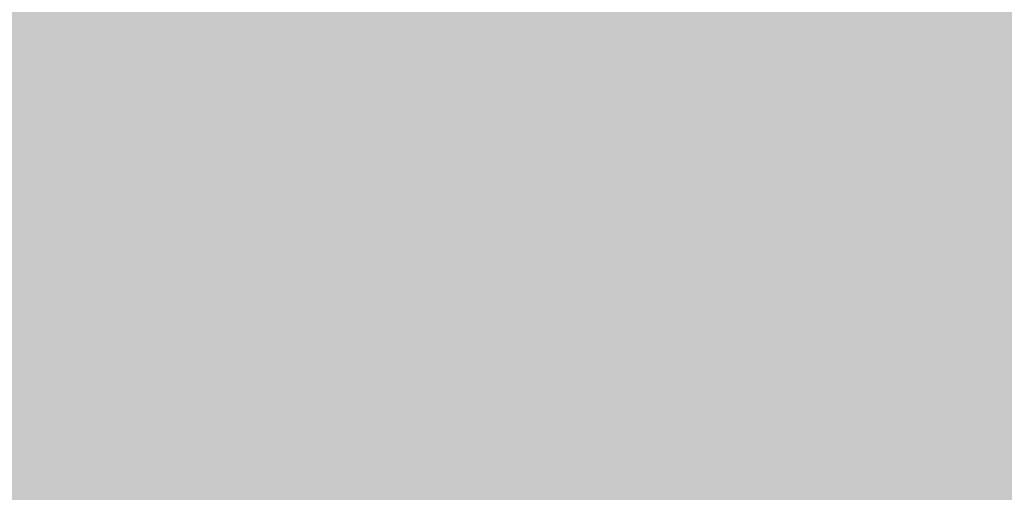
# Model space of a CAD drawing. Units: inches. Extents: x 2083 to 3317, y 1141 to 2115.
# Tile 131 of 256: x 3119.674 to 3123.979, y 1265.165 to 1267.234. Entities that reach past the tile are written whole.
import ezdxf

# ---------------------------------------------------------------- set-up
doc = ezdxf.new("R2010")
doc.units = ezdxf.units.IN
doc.layers.add('A-ANNO-DIMS', color=2, linetype='Continuous', lineweight=18)
doc.layers.add('A-WALL-PATT', color=251, linetype='Continuous', lineweight=13, true_color=0x636466)
doc.styles.get("Standard").update_dxf_attribs({"font": 'arial.ttf'})
doc.dimstyles.new('ISO-25', dxfattribs={"dimtxt": 12, "dimasz": 12, "dimexe": 1.25, "dimexo": 0.625, "dimtad": 1, "dimlunit": 3, "dimtxsty": 'Standard', "dimcen": 2.5, "dimadec": 0, "dimazin": 0, "dimtfac": 1, "dimtmove": 0, "dimatfit": 3, "dimfxl": 1, "dimarcsym": 0})

# ---------------------------------------------------------------- blocks, each defined once
blk = doc.blocks.new('*D26')
at = {"layer": 'A-ANNO-DIMS', "color": 0, "lineweight": -2, "transparency": 16777216}
for p, q in [((3088.9858, 1274.9151), (3088.9858, 1270.952)), ((3111.24, 1274.9151), (3111.24, 1270.952)), ((3076.9858, 1272.202), (2840.2624, 1272.202)), ((3111.24, 1272.202), (3088.9858, 1272.202)), ((3123.24, 1272.202), (3135.24, 1272.202))]:
    blk.add_line(p, q, dxfattribs=at)
at = {"layer": 'A-ANNO-DIMS', "color": 0, "transparency": 16777216}
for points in [[(3076.9858, 1274.202), (3076.9858, 1270.202), (3088.9858, 1272.202)], [(3123.24, 1274.202), (3123.24, 1270.202), (3111.24, 1272.202)]]:
    blk.add_solid(points, dxfattribs=at)
at = {"layer": 'Defpoints', "color": 0, "transparency": 16777216}
for p in [(3088.9858, 1275.5401), (3111.24, 1275.5401), (3088.9858, 1272.202)]:
    blk.add_point(p, dxfattribs=at)
at = {"layer": 'A-ANNO-DIMS', "color": 0, "transparency": 16777216, "insert": (2952.6241, 1279.0316), "char_height": 12, "attachment_point": 5}
blk.add_mtext('NIGHTSTAND 1\'-10 1/2" TYP.', dxfattribs=at)
blk = doc.blocks.new('*D27')
at = {"layer": 'A-ANNO-DIMS', "color": 0, "lineweight": -2, "transparency": 16777216}
for p, q in [((3114.5782, 1309.7943), (3114.5782, 1321.7943)), ((3111.865, 1297.7943), (3115.8282, 1297.7943)), ((3114.5782, 1297.7943), (3114.5782, 1275.5401)), ((3111.865, 1275.5401), (3115.8282, 1275.5401)), ((3114.5782, 1263.5401), (3114.5782, 1140.9886))]:
    blk.add_line(p, q, dxfattribs=at)
at = {"layer": 'A-ANNO-DIMS', "color": 0, "transparency": 16777216}
for points in [[(3112.5782, 1309.7943), (3116.5782, 1309.7943), (3114.5782, 1297.7943)], [(3112.5782, 1263.5401), (3116.5782, 1263.5401), (3114.5782, 1275.5401)]]:
    blk.add_solid(points, dxfattribs=at)
at = {"layer": 'Defpoints', "color": 0, "transparency": 16777216}
for p in [(3111.24, 1297.7943), (3111.24, 1275.5401), (3114.5782, 1275.5401)]:
    blk.add_point(p, dxfattribs=at)
at = {"layer": 'A-ANNO-DIMS', "color": 0, "transparency": 16777216, "insert": (3107.7485, 1196.2643), "char_height": 12, "attachment_point": 5, "rotation": 90}
blk.add_mtext('1\'-10 1/2" TYP.', dxfattribs=at)

msp = doc.modelspace()

# ---------------------------------------------------------------- hatches: boundary and pattern name
at = {"layer": 'A-WALL-PATT'}
h = msp.add_hatch(color=256, dxfattribs=at)
h.dxf.hatch_style = 1
h.paths.add_polyline_path([(3126.9598, 2020.7614), (2748.9598, 2020.7614), (2604.9598, 2020.7614), (2226.9598, 2020.7614), (2226.9598, 1702.7614), (2466.9598, 1702.7614), (2466.9598, 1582.7614), (2418.9598, 1582.7614), (2418.9598, 1477.7614), (2226.9598, 1477.7614), (2226.9598, 1263.2614), (2544.9598, 1263.2614), (2544.9598, 1411.7614), (2604.9598, 1411.7614), (2685.9598, 1411.7614), (2685.9598, 1420.7614), (2604.9598, 1420.7614), (2604.9598, 1573.7614), (2604.9598, 1702.7614), (2604.9598, 2011.7614), (2748.9598, 2011.7614), (2748.9598, 1702.7614), (2862.9598, 1702.7614), (2862.9598, 1621.7614), (2871.9598, 1621.7614), (2871.9598, 1702.7614), (2883.9598, 1702.7614), (2883.9598, 1706.9395, -0.026459), (2883.9598, 1711.7614), (2757.9598, 1711.7614), (2757.9598, 1807.7614), (2787.9598, 1807.7614), (2787.9598, 1812.2614), (2757.9598, 1812.2614), (2757.9598, 2011.7614), (2877.9598, 2011.7614), (2877.9598, 1812.2614), (2847.9598, 1812.2614), (2847.9598, 1807.7614), (2889.8357, 1807.7614), (2889.8357, 1812.2614), (2882.4598, 1812.2614), (2882.4598, 2011.7614), (3117.9598, 2011.7614), (3117.9598, 1812.2614), (2937.8357, 1812.2614), (2937.8357, 1807.7614), (2995.7098, 1807.7614), (2995.7098, 1796.1177), (3000.2098, 1796.1177), (3000.2098, 1807.7614), (3117.9598, 1807.7614), (3117.9598, 1711.7614), (3000.2098, 1711.7614), (3000.2098, 1760.1177), (2998.5727, 1760.1177, -0.020711), (2995.7098, 1760.1177), (2995.7098, 1711.7614), (2931.9598, 1711.7614), (2931.9598, 1702.7614), (3126.9598, 1702.7614)])
h.paths.add_polyline_path([(2471.4598, 2011.7614), (2471.4598, 1810.0114), (2462.7169, 1810.0114), (2462.7169, 1805.5114), (2505.9598, 1805.5114), (2505.9598, 1810.0114), (2475.9598, 1810.0114), (2475.9598, 2011.7614), (2595.9598, 2011.7614), (2595.9598, 1810.0114), (2565.9598, 1810.0114), (2565.9598, 1805.5114), (2595.9598, 1805.5114), (2595.9598, 1711.7614), (2235.9598, 1711.7614), (2235.9598, 1805.5114), (2353.7098, 1805.5114), (2353.7098, 1796.0542), (2358.2098, 1796.0542), (2358.2098, 1805.5114), (2414.7169, 1805.5114), (2414.7169, 1810.0114), (2235.9598, 1810.0114), (2235.9598, 2011.7614)], flags=16)
h.paths.add_polyline_path([(2270.2047, 1994.61), (2270.2047, 1970.61), (2246.2047, 1970.61), (2246.2047, 1994.61)], flags=0)
edge = h.paths.add_edge_path(flags=0)
edge.add_ellipse((2332.0274, 1899.7982), major_axis=(-3.043, 3.043), ratio=0.168252, start_angle=-161.3322, end_angle=-156.3071, ccw=False)
edge.add_ellipse((2333.082, 1898.7435), major_axis=(-1.0546, 1.0546), ratio=0.453532, start_angle=-123.371, end_angle=-94.1591)
edge = h.paths.add_edge_path(flags=0)
edge.add_ellipse((2332.0274, 1968.8763), major_axis=(3.043, 3.043), ratio=0.168252, start_angle=18.6678, end_angle=23.6929)
edge.add_spline(control_points=[(2332.9256, 1970.6911), (2332.2268, 1970.3361), (2330.8937, 1969.6589), (2328.4131, 1970.9321), (2327.2039, 1967.7487), (2324.7096, 1969.9556), (2322.5328, 1967.0124), (2320.0128, 1971.2958), (2317.6803, 1968.1578), (2316.0405, 1967.102), (2315.4269, 1966.8096)], knot_values=[0, 0, 0, 0, 2.267059, 4.324559, 6.685584, 8.878641, 11.121502, 14.300359, 17.755284, 19.732645, 19.732645, 19.732645, 19.732645], degree=3, periodic=0)
edge.add_ellipse((2332.0274, 1968.8763), major_axis=(3.043, 3.043), ratio=0.168252, start_angle=18.6678, end_angle=23.6929, ccw=False)
edge.add_ellipse((2333.082, 1969.9309), major_axis=(1.0546, 1.0546), ratio=0.453532, start_angle=56.629, end_angle=85.8409, ccw=False)
edge = h.paths.add_edge_path(flags=0)
edge.add_spline(control_points=[(2296.4283, 1967.9879), (2293.6278, 1965.3363), (2287.7036, 1959.7271), (2299.7439, 1949.9957), (2294.5326, 1935.6685), (2290.5732, 1920.6035), (2293.3941, 1909.9737), (2296.1854, 1904.9665)], knot_values=[0.099185, 0.099185, 0.099185, 0.099185, 0.345301, 0.619822, 0.982653, 1.386093, 1.810555, 1.810555, 1.810555, 1.810555], degree=3, periodic=0)
edge.add_spline(control_points=[(2296.1854, 1904.9665), (2297.3836, 1902.6193), (2298.001, 1901.9493), (2298.553, 1901.4682)], knot_values=[0.006246, 0.006246, 0.006246, 0.006246, 0.055476, 0.055476, 0.055476, 0.055476], degree=3, periodic=0)
edge.add_spline(control_points=[(2298.553, 1901.4682), (2297.2586, 1900.9232), (2295.2253, 1900.2321), (2293.0602, 1900.6142), (2292.1014, 1900.7884), (2292.0896, 1900.7906)], knot_values=[0.312835, 0.312835, 0.312835, 0.312835, 0.40178, 0.474987, 0.475903, 0.475903, 0.475903, 0.475903], degree=3, periodic=0)
edge.add_arc((2292.7936, 1904.6641), 3.937, 215.4209, 259.6982, ccw=False)
edge.add_spline(control_points=[(2289.5853, 1902.3823), (2289.4767, 1902.5351), (2289.3685, 1902.688), (2289.2609, 1902.8412)], knot_values=[0.102872, 0.102872, 0.102872, 0.102872, 0.116896, 0.116896, 0.116896, 0.116896], degree=3, periodic=0)
edge.add_spline(control_points=[(2289.2609, 1902.8412), (2288.6866, 1902.5502), (2287.64, 1902.0199), (2285.8813, 1901.874), (2283.853, 1901.5044), (2281.72, 1899.7105), (2278.467, 1899.4929), (2276.1571, 1901.8832), (2272.259, 1899.8041), (2267.7776, 1901.8432), (2262.2439, 1900.184), (2257.4149, 1901.7821), (2254.3184, 1900.7261), (2253.1783, 1900.3373)], knot_values=[0, 0, 0, 0, 1.907977, 3.477176, 5.261074, 7.972851, 11.680248, 13.717921, 16.939592, 22.789562, 27.502503, 33.595215, 37.145618, 37.145618, 37.145618, 37.145618], degree=3, periodic=0)
edge.add_line((2253.1783, 1900.3373), (2250.2442, 1902.8412))
edge.add_line((2250.2442, 1902.8412), (2250.2442, 1965.8333))
edge.add_line((2250.2442, 1965.8333), (2253.1783, 1968.3371))
edge.add_spline(control_points=[(2253.1783, 1968.3371), (2254.3184, 1967.9483), (2257.4149, 1966.8924), (2262.2439, 1968.4904), (2267.7776, 1966.8313), (2271.5267, 1968.5372), (2273.8759, 1967.8283), (2274.2067, 1967.7276)], knot_values=[0, 0, 0, 0, 0.09018, 0.244935, 0.364644, 0.513233, 0.537855, 0.537855, 0.537855, 0.537855], degree=3, periodic=0)
edge.add_arc((2274.3529, 1963.7933), 3.937, 72.0511, 92.1279, ccw=False)
edge.add_arc((2281.2969, 1985.23), 18.5963, 252.05113, 288.56572)
edge.add_arc((2292.3167, 1956.0289), 12.6461, 71.02679, 113.77822, ccw=False)
edge = h.paths.add_edge_path(flags=0)
edge.add_spline(control_points=[(2274.8994, 1951.8562), (2275.0662, 1951.6166), (2275.2327, 1951.3766), (2275.398, 1951.1359)], knot_values=[1.409916, 1.409916, 1.409916, 1.409916, 1.43159, 1.43159, 1.43159, 1.43159], degree=3, periodic=0)
edge.add_spline(control_points=[(2275.398, 1951.1359), (2275.7921, 1950.5619), (2276.1792, 1949.9838), (2276.5455, 1949.3971)], knot_values=[1.358238, 1.358238, 1.358238, 1.358238, 1.409916, 1.409916, 1.409916, 1.409916], degree=3, periodic=0)
edge.add_line((2276.5455, 1949.3971), (2277.4373, 1947.8622))
edge.add_spline(control_points=[(2277.4373, 1947.8622), (2276.3038, 1945.6731), (2274.6397, 1942.4269), (2274.6316, 1938.0939), (2272.7991, 1930.8515), (2274.3564, 1943.897), (2275.9477, 1947.9234), (2276.5455, 1949.3971)], knot_values=[0.005632, 0.005632, 0.005632, 0.005632, 0.186014, 0.266002, 0.357087, 0.59639, 0.739732, 0.739732, 0.739732, 0.739732], degree=3, periodic=0)
edge.add_spline(control_points=[(2276.5455, 1949.3971), (2276.1792, 1949.9838), (2275.7921, 1950.5619), (2275.398, 1951.1359)], knot_values=[1.358238, 1.358238, 1.358238, 1.358238, 1.409916, 1.409916, 1.409916, 1.409916], degree=3, periodic=0)
edge.add_spline(control_points=[(2275.398, 1951.1359), (2274.9425, 1950.0805), (2274.2078, 1948.0253), (2273.9346, 1944.8515), (2272.4685, 1937.6275), (2273.4662, 1945.6965), (2274.7006, 1951.0595), (2274.8994, 1951.8562)], knot_values=[0.104364, 0.104364, 0.104364, 0.104364, 0.189636, 0.269624, 0.36071, 0.600013, 0.644622, 0.644622, 0.644622, 0.644622], degree=3, periodic=0)
h.paths.add_polyline_path([(2269.1675, 1963.1276, -0.357527), (2268.1706, 1960.9764, -0.092561), (2268.1706, 1939.4363, -0.357527), (2269.1675, 1937.2851, -0.357527), (2267.0163, 1938.282, -0.164785), (2254.6856, 1938.282, -0.357527), (2252.5344, 1937.2851, -0.357527), (2253.5313, 1939.4363, -0.092561), (2253.5313, 1960.9764, -0.357527), (2252.5344, 1963.1276, -0.357527), (2254.6856, 1962.1307, -0.164785), (2267.0163, 1962.1307, -0.357527)], flags=0)
h.paths.add_polyline_path([(2248.8741, 1967.8018), (2248.8741, 1957.0277), (2249.4578, 1957.0277), (2249.4578, 1911.6468), (2248.8741, 1911.6468), (2248.8741, 1900.8727), (2246.5119, 1900.8727, 0.197327), (2244.1497, 1902.4569), (2244.1497, 1966.2176, 0.197327), (2246.5119, 1967.8018)], flags=0)
h.paths.add_polyline_path([(2269.1675, 1931.3893, -0.357527), (2268.1706, 1929.2381, -0.092561), (2268.1706, 1907.6981, -0.357527), (2269.1675, 1905.5469, -0.357527), (2267.0163, 1906.5438, -0.164785), (2254.6856, 1906.5438, -0.357527), (2252.5344, 1905.5469, -0.357527), (2253.5313, 1907.6981, -0.092561), (2253.5313, 1929.2381, -0.357527), (2252.5344, 1931.3893, -0.357527), (2254.6856, 1930.3925, -0.164785), (2267.0163, 1930.3925, -0.357527)], flags=0)
edge = h.paths.add_edge_path(flags=0)
edge.add_spline(control_points=[(2276.1969, 1906.7237), (2276.1681, 1909.0289), (2276.114, 1913.3719), (2270.5984, 1924.925), (2273.9052, 1919.0128), (2275.9217, 1916.2621), (2275.4746, 1912.4021), (2277.2579, 1910.3806), (2276.696, 1908.225), (2276.6462, 1906.813), (2276.6178, 1906.0084)], knot_values=[0, 0, 0, 0, 8.61026, 16.221274, 18.843057, 23.804898, 27.440828, 29.356102, 31.203478, 33.650687, 33.650687, 33.650687, 33.650687], degree=3, periodic=0)
edge.add_spline(control_points=[(2276.6178, 1906.0084), (2276.6233, 1905.6241), (2276.4977, 1904.6287), (2275.4418, 1903.8547), (2274.9373, 1903.0804), (2274.8591, 1902.8412)], knot_values=[0.156488, 0.156488, 0.156488, 0.156488, 0.184398, 0.231376, 0.250598, 0.250598, 0.250598, 0.250598], degree=3, periodic=0)
edge.add_line((2274.8591, 1902.8412), (2276.506, 1902.8412))
edge.add_spline(control_points=[(2276.506, 1902.8412), (2276.7883, 1903.0849), (2277.6651, 1904.1252), (2278.2495, 1904.3407), (2277.6539, 1908.5274), (2278.1557, 1906.2278), (2278.1005, 1905.2859), (2278.8467, 1904.069), (2277.8568, 1903.4149), (2277.8742, 1902.991), (2277.9036, 1902.8412)], knot_values=[0.059574, 0.059574, 0.059574, 0.059574, 0.080753, 0.103741, 0.16972, 0.176036, 0.207137, 0.240474, 0.262341, 0.27366, 0.27366, 0.27366, 0.27366], degree=3, periodic=0)
edge.add_line((2277.9036, 1902.8412), (2280.0298, 1902.8412))
edge.add_spline(control_points=[(2280.0298, 1902.8412), (2279.8882, 1903.0884), (2279.4993, 1903.9816), (2280.1523, 1905.9393), (2278.1036, 1909.6578), (2279.7624, 1907.1853), (2280.3279, 1904.8749), (2280.4851, 1903.4896), (2281.4633, 1903.2494), (2281.7583, 1902.9365), (2281.834, 1902.8412)], knot_values=[0.013856, 0.013856, 0.013856, 0.013856, 0.034874, 0.088867, 0.107879, 0.126738, 0.158714, 0.193757, 0.217487, 0.226722, 0.226722, 0.226722, 0.226722], degree=3, periodic=0)
edge.add_spline(control_points=[(2281.834, 1902.8412), (2281.7875, 1902.8267), (2281.647, 1902.783), (2281.3955, 1902.8595), (2281.0881, 1902.9852), (2280.7207, 1903.0609), (2280.3335, 1903.0257), (2280.1248, 1902.8989), (2280.0298, 1902.8412)], knot_values=[0, 0, 0, 0, 0.14413, 0.435517, 0.749276, 1.153046, 1.548371, 1.878348, 1.878348, 1.878348, 1.878348], degree=3, periodic=0)
edge.add_line((2280.0298, 1902.8412), (2277.9036, 1902.8412))
edge.add_spline(control_points=[(2277.9036, 1902.8412), (2277.8929, 1902.7959), (2277.8654, 1902.6796), (2277.6075, 1902.6875), (2277.2741, 1902.8007), (2276.8379, 1902.6198), (2276.5838, 1902.7893), (2276.506, 1902.8412)], knot_values=[0, 0, 0, 0, 0.127189, 0.326199, 0.628009, 1.24357, 1.515331, 1.515331, 1.515331, 1.515331], degree=3, periodic=0)
edge.add_line((2276.506, 1902.8412), (2274.8591, 1902.8412))
edge.add_spline(control_points=[(2274.8591, 1902.8412), (2274.8144, 1902.8986), (2274.7251, 1903.0134), (2274.4935, 1903.119), (2274.2443, 1902.9605), (2273.9371, 1903.1849), (2273.614, 1902.9831), (2273.4083, 1902.883), (2273.3223, 1902.8412)], knot_values=[0, 0, 0, 0, 0.21843, 0.436957, 0.687977, 0.990379, 1.398396, 1.69185, 1.69185, 1.69185, 1.69185], degree=3, periodic=0)
edge.add_spline(control_points=[(2273.3223, 1902.8412), (2273.6167, 1903.4457), (2274.274, 1904.5383), (2276.0272, 1904.5737), (2276.207, 1906.5836), (2276.1969, 1906.7237)], knot_values=[0.012227, 0.012227, 0.012227, 0.012227, 0.059472, 0.106218, 0.134458, 0.134458, 0.134458, 0.134458], degree=3, periodic=0)
h.paths.add_polyline_path([(2270.7761, 1897.7898), (2270.7761, 1873.7898), (2246.7761, 1873.7898), (2246.7761, 1897.7898)], flags=0)
h.paths.add_polyline_path([(2353.7098, 1760.0051), (2353.7098, 1760.0542), (2358.2098, 1760.0542, -0.033729)], flags=0)
h.paths.add_polyline_path([(2321.8191, 1737.5292), (2341.9953, 1737.5292, -0.414214), (2343.2033, 1736.3212), (2343.2033, 1721.0206, -0.414214), (2341.9953, 1719.8127), (2321.8191, 1719.8127, -0.414214), (2320.6112, 1721.0206), (2320.6112, 1736.3212, -0.414214)], flags=0)
h.paths.add_polyline_path([(2324.235, 1736.3212), (2339.5794, 1736.3212, -0.414214), (2341.9953, 1733.9053), (2341.9953, 1725.4497, -0.414214), (2339.5794, 1723.0338), (2333.6806, 1723.0338), (2333.8453, 1722.0455, -0.870646), (2335.4254, 1721.8259, -0.767327), (2333.9227, 1721.4232), (2331.291, 1721.4232, -0.767327), (2329.7883, 1721.8259, -0.870646), (2331.3684, 1722.0455), (2331.5331, 1723.0338), (2324.235, 1723.0338, -0.414214), (2321.8191, 1725.4497), (2321.8191, 1733.9053, -0.414214)], flags=0)
h.paths.add_polyline_path([(2570.4838, 1928.6154), (2589.6838, 1928.6154), (2590.1688, 1928.6154), (2590.1688, 1904.9934), (2570.4838, 1904.9934)], flags=0)
h.paths.add_polyline_path([(2574.4473, 1927.2638, -1), (2572.8288, 1927.2638, -1)], flags=0)
h.paths.add_polyline_path([(2573.0899, 1926.9409), (2573.925, 1927.776), (2574.1477, 1927.5533), (2573.3126, 1926.7182)], flags=0)
h.paths.add_polyline_path([(2578.7791, 1919.7296, -1), (2571.5917, 1919.7296, -1)], flags=0)
h.paths.add_polyline_path([(2578.3854, 1919.7296, -1), (2571.9854, 1919.7296, -1)], flags=0)
h.paths.add_polyline_path([(2331.5958, 1729.4762, -1), (2333.618, 1729.4762, -1)], flags=0)
h.paths.add_polyline_path([(2578.0342, 1927.2638, -1), (2576.4157, 1927.2638, -1)], flags=0)
h.paths.add_polyline_path([(2576.6889, 1927.5311), (2576.9116, 1927.7538), (2577.7467, 1926.9186), (2577.524, 1926.6959)], flags=0)
h.paths.add_polyline_path([(2578.1391, 1909.8595, -1), (2572.2317, 1909.8595, -1)], flags=0)
h.paths.add_polyline_path([(2577.7454, 1909.8595, -1), (2572.6254, 1909.8595, -1)], flags=0)
h.paths.add_polyline_path([(2583.7977, 1927.2638, -1), (2582.1792, 1927.2638, -1)], flags=0)
h.paths.add_polyline_path([(2582.7186, 1927.7538), (2583.5538, 1926.9186), (2583.3311, 1926.6959), (2582.4959, 1927.5311)], flags=0)
h.paths.add_polyline_path([(2582.4959, 1927.5311), (2582.7186, 1927.7538), (2583.5538, 1926.9186), (2583.3311, 1926.6959)], flags=0)
h.paths.add_polyline_path([(2587.7391, 1920.5296, -1), (2581.8317, 1920.5296, -1)], flags=0)
h.paths.add_polyline_path([(2587.3454, 1920.5296, -1), (2582.2254, 1920.5296, -1)], flags=0)
h.paths.add_polyline_path([(2587.3846, 1927.2638, -1), (2585.7661, 1927.2638, -1)], flags=0)
h.paths.add_polyline_path([(2586.082, 1926.9802), (2586.9172, 1927.8154), (2587.1399, 1927.5927), (2586.3047, 1926.7575)], flags=0)
h.paths.add_polyline_path([(2588.3791, 1910.6595, -1), (2581.1917, 1910.6595, -1)], flags=0)
h.paths.add_polyline_path([(2587.9854, 1910.6595, -1), (2581.5854, 1910.6595, -1)], flags=0)
h.paths.add_polyline_path([(2417.1677, 1729.4779), (2437.3439, 1729.4779, -0.414214), (2438.5519, 1728.2699), (2438.5519, 1712.9693, -0.414214), (2437.3439, 1711.7614), (2417.1677, 1711.7614, -0.414214), (2415.9598, 1712.9693), (2415.9598, 1728.2699, -0.414214)], flags=0)
h.paths.add_polyline_path([(2419.5836, 1728.2699), (2434.928, 1728.2699, -0.414214), (2437.3439, 1725.8541), (2437.3439, 1717.3984, -0.414214), (2434.928, 1714.9825), (2429.0292, 1714.9825), (2429.1939, 1713.9942, -0.870646), (2430.774, 1713.7746, -0.767327), (2429.2713, 1713.372), (2426.6396, 1713.372, -0.767327), (2425.1369, 1713.7746, -0.870646), (2426.717, 1713.9942), (2426.8817, 1714.9825), (2419.5836, 1714.9825, -0.414214), (2417.1677, 1717.3984), (2417.1677, 1725.8541, -0.414214)], flags=0)
h.paths.add_polyline_path([(2419.5836, 1728.2699), (2434.928, 1728.2699, -0.414214), (2437.3439, 1725.8541), (2437.3439, 1717.3984, -0.414214), (2434.928, 1714.9825), (2429.0292, 1714.9825), (2428.3581, 1719.009), (2427.5528, 1719.009), (2426.8817, 1714.9825), (2419.5836, 1714.9825, -0.414214), (2417.1677, 1717.3984), (2417.1677, 1725.8541, -0.414214)], flags=0)
h.paths.add_polyline_path([(2426.9444, 1721.4249, -1), (2428.9666, 1721.4249, -1)], flags=0)
h.paths.add_polyline_path([(2475.9598, 1702.7614), (2595.9598, 1702.7614), (2595.9598, 1582.7614), (2475.9598, 1582.7614)], flags=16)
h.paths.add_polyline_path([(2427.9598, 1573.7614), (2595.9598, 1573.7614), (2595.9598, 1468.7614), (2595.9598, 1420.7614), (2384.4598, 1420.7614), (2384.4598, 1468.7614), (2427.9598, 1468.7614)], flags=16)
h.paths.add_polyline_path([(2379.9598, 1468.7614), (2379.9598, 1420.7614), (2235.9598, 1420.7614), (2235.9598, 1468.7614)], flags=16)
h.paths.add_polyline_path([(2317.816, 1466.6958), (2337.9922, 1466.6958, -0.414214), (2339.2002, 1465.4878), (2339.2002, 1450.1872, -0.414214), (2337.9922, 1448.9792), (2317.816, 1448.9792, -0.414214), (2316.6081, 1450.1872), (2316.6081, 1465.4878, -0.414214)], flags=0)
h.paths.add_polyline_path([(2320.2319, 1465.4878), (2335.5763, 1465.4878, -0.414214), (2337.9922, 1463.0719), (2337.9922, 1454.6163, -0.414214), (2335.5763, 1452.2004), (2329.6775, 1452.2004), (2329.8422, 1451.212, -0.870646), (2331.4223, 1450.9925, -0.767327), (2329.9196, 1450.5898), (2327.2879, 1450.5898, -0.767327), (2325.7852, 1450.9925, -0.870646), (2327.3653, 1451.212), (2327.53, 1452.2004), (2320.2319, 1452.2004, -0.414214), (2317.816, 1454.6163), (2317.816, 1463.0719, -0.414214)], flags=0)
h.paths.add_polyline_path([(2320.2319, 1465.4878), (2335.5763, 1465.4878, -0.414214), (2337.9922, 1463.0719), (2337.9922, 1454.6163, -0.414214), (2335.5763, 1452.2004), (2329.6775, 1452.2004), (2329.0064, 1456.2269), (2328.2011, 1456.2269), (2327.53, 1452.2004), (2320.2319, 1452.2004, -0.414214), (2317.816, 1454.6163), (2317.816, 1463.0719, -0.414214)], flags=0)
h.paths.add_polyline_path([(2327.5926, 1458.6428, -1), (2329.6148, 1458.6428, -1)], flags=0)
h.paths.add_polyline_path([(2244.4117, 1433.3405), (2241.9209, 1433.3405, -0.414214), (2240.0179, 1435.2435), (2240.0179, 1440.9528, -0.414211), (2241.9209, 1442.8559), (2244.4117, 1442.8559, -1.976472)], flags=0)
h.paths.add_polyline_path([(2245.3569, 1434.3975, -0.414214), (2245.3569, 1441.7988, -2.144098)], flags=0)
h.paths.add_polyline_path([(2535.9598, 1416.2614), (2535.9598, 1272.2614), (2235.9598, 1272.2614), (2235.9598, 1416.2614)], flags=16)
h.paths.add_polyline_path([(2260.1196, 1384.2928), (2260.1196, 1362.0386), (2237.8654, 1362.0386), (2237.8654, 1384.2928)], flags=0)
edge = h.paths.add_edge_path(flags=0)
edge.add_line((2318.2518, 1362.0933), (2318.1458, 1362.001))
edge.add_ellipse((2317.4451, 1360.431), major_axis=(2.8216, 2.8216), ratio=0.168252, start_angle=18.6678, end_angle=20.9481, ccw=False)
edge.add_ellipse((2318.423, 1361.409), major_axis=(0.9779, 0.9779), ratio=0.453532, start_angle=56.629, end_angle=70.2262, ccw=False)
edge = h.paths.add_edge_path(flags=0)
edge.add_line((2319.1074, 1295.5711), (2319.015, 1295.6771))
edge.add_ellipse((2317.4451, 1296.3778), major_axis=(-2.8216, 2.8216), ratio=0.168252, start_angle=-161.3322, end_angle=-159.0519, ccw=False)
edge.add_ellipse((2318.423, 1295.3999), major_axis=(-0.9779, 0.9779), ratio=0.453532, start_angle=-123.371, end_angle=-109.7738)
edge = h.paths.add_edge_path(flags=0)
edge.add_spline(control_points=[(2284.2103, 1301.1702), (2284.5807, 1300.4447), (2284.8912, 1299.892), (2285.1596, 1299.461)], knot_values=[0.039066, 0.039066, 0.039066, 0.039066, 0.055476, 0.055476, 0.055476, 0.055476], degree=3, periodic=0)
edge.add_line((2285.1596, 1299.461), (2284.2103, 1301.1702))
edge = h.paths.add_edge_path(flags=0)
edge.add_line((2280.4125, 1297.298), (2283.37, 1297.0361))
edge.add_line((2283.37, 1297.0361), (2286.4057, 1297.9263))
edge.add_spline(control_points=[(2286.4057, 1297.9263), (2285.3055, 1297.4631), (2284.3448, 1297.1292), (2283.37, 1297.0361)], knot_values=[0.394369, 0.394369, 0.394369, 0.394369, 0.475903, 0.475903, 0.475903, 0.475903], degree=3, periodic=0)
edge.add_spline(control_points=[(2283.37, 1297.0361), (2283.2814, 1297.0277), (2282.3163, 1296.9573), (2281.3125, 1297.1345), (2280.4234, 1297.296), (2280.4125, 1297.298)], knot_values=[0.312835, 0.312835, 0.312835, 0.312835, 0.320246, 0.393453, 0.394369, 0.394369, 0.394369, 0.394369], degree=3, periodic=0)
edge = h.paths.add_edge_path(flags=0)
edge.add_line((2284.4356, 1359.6073), (2280.4463, 1355.328))
edge.add_line((2280.4463, 1355.328), (2279.58, 1351.0178))
edge.add_line((2279.58, 1351.0178), (2282.413, 1346.5804))
edge.add_spline(control_points=[(2282.413, 1346.5804), (2283.1533, 1345.5892), (2284.2529, 1344.0289), (2284.801, 1342.3872), (2284.9352, 1341.8055)], knot_values=[1.240098, 1.240098, 1.240098, 1.240098, 1.332892, 1.382712, 1.382712, 1.382712, 1.382712], degree=3, periodic=0)
edge.add_spline(control_points=[(2284.9352, 1341.8055), (2285.3191, 1340.1406), (2285.233, 1338.4092), (2284.9099, 1336.6541)], knot_values=[1.097484, 1.097484, 1.097484, 1.097484, 1.240098, 1.240098, 1.240098, 1.240098], degree=3, periodic=0)
edge.add_spline(control_points=[(2284.9099, 1336.6541), (2284.5868, 1334.899), (2284.0267, 1333.1203), (2283.4626, 1331.3606)], knot_values=[0.95487, 0.95487, 0.95487, 0.95487, 1.097484, 1.097484, 1.097484, 1.097484], degree=3, periodic=0)
edge.add_line((2283.4626, 1331.3606), (2281.8904, 1326.1534))
edge.add_line((2281.8904, 1326.1534), (2280.7563, 1321.0561))
edge.add_line((2280.7563, 1321.0561), (2280.2992, 1316.002))
edge.add_line((2280.2992, 1316.002), (2280.7159, 1310.9501))
edge.add_line((2280.7159, 1310.9501), (2282.0281, 1305.9721))
edge.add_line((2282.0281, 1305.9721), (2284.2103, 1301.1702))
edge.add_spline(control_points=[(2284.2103, 1301.1702), (2283.3407, 1302.7302), (2282.6119, 1304.3365), (2282.0281, 1305.9721)], knot_values=[0.099185, 0.099185, 0.099185, 0.099185, 0.241799, 0.241799, 0.241799, 0.241799], degree=3, periodic=0)
edge.add_spline(control_points=[(2282.0281, 1305.9721), (2281.4443, 1307.6078), (2281.0055, 1309.2728), (2280.7159, 1310.9501)], knot_values=[0.241799, 0.241799, 0.241799, 0.241799, 0.384413, 0.384413, 0.384413, 0.384413], degree=3, periodic=0)
edge.add_spline(control_points=[(2280.7159, 1310.9501), (2280.4332, 1312.5876), (2280.2894, 1314.277), (2280.2989, 1315.962), (2280.2992, 1316.002)], knot_values=[0.384413, 0.384413, 0.384413, 0.384413, 0.523647, 0.527028, 0.527028, 0.527028, 0.527028], degree=3, periodic=0)
edge.add_spline(control_points=[(2280.2992, 1316.002), (2280.3123, 1317.687), (2280.4779, 1319.3679), (2280.7563, 1321.0561)], knot_values=[0.527028, 0.527028, 0.527028, 0.527028, 0.669642, 0.669642, 0.669642, 0.669642], degree=3, periodic=0)
edge.add_spline(control_points=[(2280.7563, 1321.0561), (2281.0346, 1322.7443), (2281.4259, 1324.4396), (2281.8904, 1326.1534)], knot_values=[0.669642, 0.669642, 0.669642, 0.669642, 0.812256, 0.812256, 0.812256, 0.812256], degree=3, periodic=0)
edge.add_spline(control_points=[(2281.8904, 1326.1534), (2282.2644, 1327.5333), (2282.7879, 1329.2618), (2283.3528, 1331.0178), (2283.4626, 1331.3606)], knot_values=[0.812256, 0.812256, 0.812256, 0.812256, 0.927087, 0.95487, 0.95487, 0.95487, 0.95487], degree=3, periodic=0)
edge.add_line((2283.4626, 1331.3606), (2284.9099, 1336.6541))
edge.add_line((2284.9099, 1336.6541), (2284.9352, 1341.8055))
edge.add_line((2284.9352, 1341.8055), (2282.413, 1346.5804))
edge.add_spline(control_points=[(2282.413, 1346.5804), (2281.2751, 1348.1038), (2280.0784, 1349.5703), (2279.58, 1351.0178)], knot_values=[1.382712, 1.382712, 1.382712, 1.382712, 1.525326, 1.525326, 1.525326, 1.525326], degree=3, periodic=0)
edge.add_spline(control_points=[(2279.58, 1351.0178), (2279.4433, 1351.4147), (2279.1363, 1352.8569), (2279.7352, 1354.2904), (2280.4463, 1355.328)], knot_values=[1.525326, 1.525326, 1.525326, 1.525326, 1.564439, 1.667941, 1.667941, 1.667941, 1.667941], degree=3, periodic=0)
edge.add_spline(control_points=[(2280.4463, 1355.328), (2281.4261, 1356.7578), (2282.9308, 1358.1826), (2284.4356, 1359.6073)], knot_values=[1.667941, 1.667941, 1.667941, 1.667941, 1.810555, 1.810555, 1.810555, 1.810555], degree=3, periodic=0)
edge.add_arc((2280.6231, 1348.5182), 11.7262, 71.02679, 113.77822)
edge.add_arc((2270.4049, 1375.5952), 17.2436, 252.05113, 288.56572, ccw=False)
edge.add_arc((2263.966, 1355.7178), 3.6506, 72.0511, 92.1279)
edge.add_arc((2263.966, 1355.7178), 3.6506, 92.1279, 177.9851)
edge.add_spline(control_points=[(2260.3176, 1355.8462), (2260.2604, 1354.2207), (2260.5513, 1350.1865), (2262.9993, 1346.7663), (2264.4727, 1344.649)], knot_values=[1.43159, 1.43159, 1.43159, 1.43159, 1.564144, 1.770695, 1.770695, 1.770695, 1.770695], degree=3, periodic=0)
edge.add_line((2264.4727, 1344.649), (2264.9356, 1343.9825))
edge.add_spline(control_points=[(2263.801, 1340.2481), (2263.8432, 1340.5141), (2264.0672, 1341.7565), (2264.5127, 1343.0025), (2264.935, 1343.9811)], knot_values=[0.53657, 0.53657, 0.53657, 0.53657, 0.559349, 0.644622, 0.644622, 0.644622, 0.644622], degree=3, periodic=0)
edge.add_spline(control_points=[(2264.935, 1343.9811), (2265.1178, 1343.715), (2265.2989, 1343.4479), (2265.4768, 1343.1794)], knot_values=[1.384077, 1.384077, 1.384077, 1.384077, 1.409916, 1.409916, 1.409916, 1.409916], degree=3, periodic=0)
edge.add_spline(control_points=[(2265.4768, 1343.1794), (2265.6546, 1342.9108), (2265.8293, 1342.6408), (2265.9991, 1342.3688)], knot_values=[1.358238, 1.358238, 1.358238, 1.358238, 1.384077, 1.384077, 1.384077, 1.384077], degree=3, periodic=0)
edge.add_line((2265.9991, 1342.3688), (2266.826, 1340.9455))
edge.add_spline(control_points=[(2266.826, 1340.9455), (2268.8944, 1337.0897), (2271.3982, 1325.843), (2270.5162, 1310.5686), (2275.9194, 1301.8606), (2277.7895, 1299.1994)], knot_values=[0.116896, 0.116896, 0.116896, 0.116896, 0.472987, 1.050969, 1.313793, 1.313793, 1.313793, 1.313793], degree=3, periodic=0)
edge.add_spline(control_points=[(2277.7895, 1299.1994), (2277.8394, 1299.1285), (2277.8894, 1299.0575), (2277.9396, 1298.9866)], knot_values=[0.109884, 0.109884, 0.109884, 0.109884, 0.116896, 0.116896, 0.116896, 0.116896], degree=3, periodic=0)
edge.add_line((2277.9396, 1298.9866), (2277.7888, 1299.1991))
edge.add_spline(control_points=[(2277.7888, 1299.1991), (2277.2566, 1298.9294), (2276.2864, 1298.4379), (2275.0394, 1298.3344), (2274.3833, 1298.2389), (2274.2153, 1298.2093)], knot_values=[33.12187, 33.12187, 33.12187, 33.12187, 35.029056, 36.598255, 37.144827, 37.144827, 37.144827, 37.144827], degree=3, periodic=0)
edge.add_line((2274.2153, 1298.2093), (2273.0731, 1297.893))
edge.add_spline(control_points=[(2273.0731, 1297.893), (2272.3229, 1297.5798), (2271.0392, 1296.5105), (2269.2484, 1296.2261), (2268.4231, 1296.3747)], knot_values=[26.532584, 26.532584, 26.532584, 26.532584, 29.198919, 31.839101, 31.839101, 31.839101, 31.839101], degree=3, periodic=0)
edge.add_line((2268.4231, 1296.3747), (2263.8785, 1297.4575))
edge.add_spline(control_points=[(2263.8785, 1297.4575), (2263.5561, 1297.3594), (2261.8603, 1296.8387), (2260.2388, 1297.2824), (2258.9335, 1297.5165)], knot_values=[15.919551, 15.919551, 15.919551, 15.919551, 16.939592, 21.226067, 21.226067, 21.226067, 21.226067], degree=3, periodic=0)
edge.add_line((2258.9335, 1297.5165), (2254.0552, 1297.329))
edge.add_spline(control_points=[(2254.0552, 1297.329), (2253.7555, 1297.2958), (2252.1137, 1297.1652), (2250.4619, 1297.5442), (2249.1297, 1297.6679)], knot_values=[5.306517, 5.306517, 5.306517, 5.306517, 6.276435, 10.613034, 10.613034, 10.613034, 10.613034], degree=3, periodic=0)
edge.add_line((2249.1297, 1297.6679), (2244.3316, 1296.8778))
edge.add_line((2244.3316, 1296.8778), (2241.611, 1299.1994))
edge.add_line((2241.611, 1299.1994), (2241.611, 1357.6094))
edge.add_line((2241.611, 1357.6094), (2244.3316, 1359.9311))
edge.add_line((2244.3316, 1359.9311), (2252.7288, 1359.5427))
edge.add_spline(control_points=[(2252.7288, 1359.5427), (2252.8709, 1359.5464), (2253.3057, 1359.5482), (2253.7398, 1359.5143), (2254.0317, 1359.4824)], knot_values=[0.233291, 0.233291, 0.233291, 0.233291, 0.244935, 0.268927, 0.268927, 0.268927, 0.268927], degree=3, periodic=0)
edge.add_line((2254.0317, 1359.4824), (2259.5872, 1359.4164))
edge.add_spline(control_points=[(2259.5872, 1359.4164), (2260.6771, 1359.6285), (2262.0732, 1359.897), (2263.5237, 1359.4593), (2263.8304, 1359.366)], knot_values=[0.422516, 0.422516, 0.422516, 0.422516, 0.513233, 0.537855, 0.537855, 0.537855, 0.537855], degree=3, periodic=0)
edge.add_arc((2263.966, 1355.7178), 3.6506, 72.0511, 92.1279, ccw=False)
edge.add_arc((2270.4049, 1375.5952), 17.2436, 252.05113, 288.56572)
edge.add_arc((2280.6231, 1348.5182), 11.7262, 71.02679, 113.77822, ccw=False)
h.paths.add_polyline_path([(2240.3405, 1359.4347), (2240.3405, 1349.4444), (2240.8818, 1349.4444), (2240.8818, 1307.3645), (2240.3405, 1307.3645), (2240.3405, 1297.3741), (2238.1502, 1297.3741, 0.197327), (2235.9598, 1298.8431), (2235.9598, 1357.9657, 0.197327), (2238.1502, 1359.4347)], flags=0)
h.paths.add_polyline_path([(2259.1578, 1355.1005, -0.357527), (2258.2334, 1353.1058, -0.092561), (2258.2334, 1333.1326, -0.357527), (2259.1578, 1331.1379, -0.357527), (2257.1631, 1332.0622, -0.164785), (2245.7293, 1332.0622, -0.357527), (2243.7346, 1331.1379, -0.357527), (2244.6589, 1333.1326, -0.092561), (2244.6589, 1353.1058, -0.357527), (2243.7346, 1355.1005, -0.357527), (2245.7293, 1354.1761, -0.164785), (2257.1631, 1354.1761, -0.357527)], flags=0)
edge = h.paths.add_edge_path(flags=0)
edge.add_line((2265.9991, 1342.3688), (2266.826, 1340.9455))
edge.add_line((2266.826, 1340.9455), (2265.3076, 1337.8141))
edge.add_line((2265.3076, 1337.8141), (2264.3582, 1334.6529))
edge.add_line((2264.3582, 1334.6529), (2264.262, 1333.7997))
edge.add_spline(control_points=[(2264.262, 1333.7997), (2264.2084, 1333.1871), (2264.1621, 1332.3655), (2264.0071, 1331.4139), (2263.969, 1331.2018)], knot_values=[0.464444, 0.464444, 0.464444, 0.464444, 0.516691, 0.531608, 0.531608, 0.531608, 0.531608], degree=3, periodic=0)
edge.add_spline(control_points=[(2263.969, 1331.2018), (2263.7745, 1330.1189), (2263.4244, 1328.7908), (2263.2574, 1328.5307), (2263.234, 1328.5146)], knot_values=[0.372682, 0.372682, 0.372682, 0.372682, 0.44885, 0.464444, 0.464444, 0.464444, 0.464444], degree=3, periodic=0)
edge.add_spline(control_points=[(2263.234, 1328.5146), (2263.0964, 1328.4202), (2263.1312, 1329.3015), (2263.275, 1330.6157)], knot_values=[0.280919, 0.280919, 0.280919, 0.280919, 0.372682, 0.372682, 0.372682, 0.372682], degree=3, periodic=0)
edge.add_spline(control_points=[(2263.275, 1330.6157), (2263.4187, 1331.93), (2263.6715, 1333.6773), (2263.9699, 1335.315)], knot_values=[0.189157, 0.189157, 0.189157, 0.189157, 0.280919, 0.280919, 0.280919, 0.280919], degree=3, periodic=0)
edge.add_spline(control_points=[(2263.9699, 1335.315), (2264.1005, 1336.0322), (2264.4188, 1337.6219), (2264.7548, 1338.8644), (2264.9474, 1339.4911)], knot_values=[0.097394, 0.097394, 0.097394, 0.097394, 0.137578, 0.189157, 0.189157, 0.189157, 0.189157], degree=3, periodic=0)
edge.add_spline(control_points=[(2264.9474, 1339.4911), (2265.29, 1340.6061), (2265.6442, 1341.494), (2265.9991, 1342.3688)], knot_values=[0.005632, 0.005632, 0.005632, 0.005632, 0.097394, 0.097394, 0.097394, 0.097394], degree=3, periodic=0)
h.paths.add_polyline_path([(2259.1578, 1325.671, -0.357527), (2258.2334, 1323.6763, -0.092561), (2258.2334, 1303.7031, -0.357527), (2259.1578, 1301.7084, -0.357527), (2257.1631, 1302.6327, -0.164785), (2245.7293, 1302.6327, -0.357527), (2243.7346, 1301.7084, -0.357527), (2244.6589, 1303.7031, -0.092561), (2244.6589, 1323.6763, -0.357527), (2243.7346, 1325.671, -0.357527), (2245.7293, 1324.7466, -0.164785), (2257.1631, 1324.7466, -0.357527)], flags=0)
edge = h.paths.add_edge_path(flags=0)
edge.add_spline(control_points=[(2261.7089, 1317.3114), (2261.6795, 1317.4176), (2261.7619, 1317.3885), (2262.4907, 1316.0899), (2262.9622, 1315.3009)], knot_values=[14.955861, 14.955861, 14.955861, 14.955861, 16.221274, 18.694826, 18.694826, 18.694826, 18.694826], degree=3, periodic=0)
edge.add_spline(control_points=[(2262.9622, 1315.3009), (2262.9904, 1315.2536), (2263.7021, 1314.0674), (2264.349, 1313.1272), (2264.7301, 1312.1642)], knot_values=[18.694826, 18.694826, 18.694826, 18.694826, 18.843057, 22.433791, 22.433791, 22.433791, 22.433791], degree=3, periodic=0)
edge.add_spline(control_points=[(2264.7301, 1312.1642), (2264.8756, 1311.7964), (2265.1769, 1310.7698), (2265.1431, 1309.5593), (2265.2477, 1308.8242)], knot_values=[22.433791, 22.433791, 22.433791, 22.433791, 23.804898, 26.172756, 26.172756, 26.172756, 26.172756], degree=3, periodic=0)
edge.add_line((2265.2477, 1308.8242), (2265.8508, 1307.1719))
edge.add_spline(control_points=[(2265.8508, 1307.1719), (2266.065, 1306.8217), (2266.3844, 1306.3322), (2266.4244, 1305.7805), (2266.4204, 1305.6112)], knot_values=[28.062562, 28.062562, 28.062562, 28.062562, 29.356102, 29.911721, 29.911721, 29.911721, 29.911721], degree=3, periodic=0)
edge.add_spline(control_points=[(2266.4204, 1305.6112), (2266.4161, 1305.4326), (2266.394, 1305.25), (2266.3648, 1305.0659)], knot_values=[29.911721, 29.911721, 29.911721, 29.911721, 30.497837, 30.497837, 30.497837, 30.497837], degree=3, periodic=0)
edge.add_line((2266.3648, 1305.0659), (2266.0662, 1302.1363))
edge.add_spline(control_points=[(2266.0662, 1302.1363), (2266.0712, 1301.78), (2265.9981, 1301.2), (2265.6633, 1300.759), (2265.5089, 1300.5859)], knot_values=[0.156488, 0.156488, 0.156488, 0.156488, 0.184398, 0.203543, 0.203543, 0.203543, 0.203543], degree=3, periodic=0)
edge.add_line((2265.5089, 1300.5859), (2264.4353, 1299.1994))
edge.add_line((2264.4353, 1299.1994), (2265.9624, 1299.1994))
edge.add_line((2265.9624, 1299.1994), (2267.336, 1301.1753))
edge.add_line((2267.336, 1301.1753), (2267.3117, 1301.9862))
edge.add_spline(control_points=[(2267.3117, 1301.9862), (2267.2611, 1302.8624), (2267.1602, 1303.7371), (2267.2715, 1303.3259)], knot_values=[0.126229, 0.126229, 0.126229, 0.126229, 0.166617, 0.166617, 0.166617, 0.166617], degree=3, periodic=0)
edge.add_spline(control_points=[(2267.2715, 1303.3259), (2267.28, 1303.2943), (2267.3098, 1303.1754), (2267.3735, 1302.8836), (2267.4061, 1302.6828), (2267.4179, 1302.601)], knot_values=[0.166617, 0.166617, 0.166617, 0.166617, 0.16972, 0.176036, 0.180765, 0.180765, 0.180765, 0.180765], degree=3, periodic=0)
edge.add_spline(control_points=[(2267.7439, 1300.9875), (2267.6876, 1301.1509), (2267.4805, 1301.6567), (2267.4838, 1302.1448), (2267.4179, 1302.601)], knot_values=[0.180765, 0.180765, 0.180765, 0.180765, 0.193767, 0.220139, 0.220139, 0.220139, 0.220139], degree=3, periodic=0)
edge.add_line((2267.4179, 1302.601), (2267.7439, 1300.9875))
edge.add_spline(control_points=[(2267.7439, 1300.9875), (2267.832, 1300.7319), (2267.932, 1300.3099), (2267.5548, 1299.9745), (2267.4294, 1299.8292)], knot_values=[0.220139, 0.220139, 0.220139, 0.220139, 0.240474, 0.25489, 0.25489, 0.25489, 0.25489], degree=3, periodic=0)
edge.add_line((2267.4294, 1299.8292), (2267.2584, 1299.1994))
edge.add_line((2267.2584, 1299.1994), (2269.23, 1299.1994))
edge.add_spline(control_points=[(2269.23, 1299.1994), (2269.0987, 1299.4287), (2268.8428, 1300.0163), (2269.0116, 1300.9159), (2268.9468, 1301.6607)], knot_values=[0.013856, 0.013856, 0.013856, 0.013856, 0.034874, 0.067073, 0.067073, 0.067073, 0.067073], degree=3, periodic=0)
edge.add_line((2268.9468, 1301.6607), (2268.4316, 1303.6031))
edge.add_spline(control_points=[(2268.4316, 1303.6031), (2268.1756, 1304.1924), (2267.5962, 1305.2513), (2268.0407, 1304.6232), (2268.2514, 1304.2824)], knot_values=[0.090155, 0.090155, 0.090155, 0.090155, 0.107879, 0.120289, 0.120289, 0.120289, 0.120289], degree=3, periodic=0)
edge.add_spline(control_points=[(2268.2514, 1304.2824), (2268.3609, 1304.1053), (2269.0578, 1302.918), (2269.3827, 1301.5904), (2269.5214, 1300.7759), (2269.5752, 1300.5558)], knot_values=[0.120289, 0.120289, 0.120289, 0.120289, 0.126738, 0.158714, 0.173506, 0.173506, 0.173506, 0.173506], degree=3, periodic=0)
edge.add_line((2269.5752, 1300.5558), (2270.6858, 1299.4213))
edge.add_spline(control_points=[(2270.6858, 1299.4213), (2270.7672, 1299.3573), (2270.8379, 1299.2814), (2270.9029, 1299.1994)], knot_values=[0.21816, 0.21816, 0.21816, 0.21816, 0.226722, 0.226722, 0.226722, 0.226722], degree=3, periodic=0)
edge.add_line((2270.9372, 1299.1929), (2270.9029, 1299.1994))
edge.add_spline(control_points=[(2270.9029, 1299.1994), (2270.8598, 1299.186), (2270.7295, 1299.1455), (2270.4963, 1299.2164), (2270.2717, 1299.3083), (2270.121, 1299.348), (2270.0633, 1299.3596)], knot_values=[0.939174, 0.939174, 0.939174, 0.939174, 1.083304, 1.374691, 1.68845, 1.878348, 1.878348, 1.878348, 1.878348], degree=3, periodic=0)
edge.add_line((2270.0633, 1299.3596), (2269.23, 1299.1994))
edge.add_line((2269.23, 1299.1994), (2267.2584, 1299.1994))
edge.add_spline(control_points=[(2267.2584, 1299.1994), (2267.2484, 1299.1574), (2267.223, 1299.0497), (2266.9838, 1299.0569), (2266.8092, 1299.1162), (2266.6769, 1299.1091), (2266.6365, 1299.1048)], knot_values=[0.757665, 0.757665, 0.757665, 0.757665, 0.884854, 1.083864, 1.385675, 1.515331, 1.515331, 1.515331, 1.515331], degree=3, periodic=0)
edge.add_spline(control_points=[(2266.6365, 1299.1048), (2266.4852, 1299.0888), (2266.2358, 1299.0171), (2266.0346, 1299.1513), (2265.9624, 1299.1994)], knot_values=[0, 0, 0, 0, 0.485905, 0.757665, 0.757665, 0.757665, 0.757665], degree=3, periodic=0)
edge.add_line((2265.9624, 1299.1994), (2264.4353, 1299.1994))
edge.add_line((2264.4353, 1299.1994), (2263.8584, 1299.3671))
edge.add_spline(control_points=[(2263.8584, 1299.3671), (2263.8189, 1299.3709), (2263.7795, 1299.3857), (2263.7401, 1299.4015)], knot_values=[0.845925, 0.845925, 0.845925, 0.845925, 0.978627, 0.978627, 0.978627, 0.978627], degree=3, periodic=0)
edge.add_line((2263.7218, 1299.3964), (2263.0103, 1299.1994))
edge.add_spline(control_points=[(2263.0103, 1299.1994), (2263.2458, 1299.6829), (2263.506, 1300.1281), (2263.8735, 1300.408)], knot_values=[0.012227, 0.012227, 0.012227, 0.012227, 0.052971, 0.052971, 0.052971, 0.052971], degree=3, periodic=0)
edge.add_spline(control_points=[(2263.8735, 1300.408), (2263.9321, 1300.4527), (2264.0842, 1300.553), (2264.2552, 1300.6242), (2264.3597, 1300.6647)], knot_values=[0.052971, 0.052971, 0.052971, 0.052971, 0.059472, 0.069086, 0.069086, 0.069086, 0.069086], degree=3, periodic=0)
edge.add_line((2264.3597, 1300.6647), (2265.1419, 1301.0778))
edge.add_line((2265.1419, 1301.0778), (2265.6758, 1302.7996))
edge.add_line((2265.6758, 1302.7996), (2265.5407, 1305.7041))
edge.add_line((2265.5407, 1305.7041), (2264.8031, 1309.3277))
edge.add_line((2264.8031, 1309.3277), (2263.0405, 1314.0918))
edge.add_spline(control_points=[(2263.0405, 1314.0918), (2262.3836, 1315.6714), (2261.796, 1316.9977), (2261.7089, 1317.3114)], knot_values=[11.216896, 11.216896, 11.216896, 11.216896, 14.955861, 14.955861, 14.955861, 14.955861], degree=3, periodic=0)
h.paths.add_polyline_path([(2871.9598, 1416.2614), (2895.91, 1416.2614), (2895.91, 1420.7614), (2871.9598, 1420.7614), (2871.9598, 1501.7614), (2862.9598, 1501.7614), (2862.9598, 1420.7614), (2805.9598, 1420.7614), (2805.9598, 1411.7614), (2862.9598, 1411.7614), (2862.9598, 1263.2614), (3126.9598, 1263.2614), (3126.9598, 1411.7614), (3126.9598, 1486.7614), (2943.9598, 1486.7614), (2943.9598, 1477.7614), (2967.8603, 1477.7614), (2967.8603, 1420.7614), (2943.91, 1420.7614), (2943.91, 1416.2614), (3117.9598, 1416.2614), (3117.9598, 1420.7614), (2972.3603, 1420.7614), (2972.3603, 1477.7614), (3117.9598, 1477.7614), (3117.9598, 1420.7614), (3117.9598, 1272.2614), (2871.9598, 1272.2614)], flags=0)
h.paths.add_polyline_path([(2457.1256, 1485.9425), (2527.6027, 1485.9425), (2527.6027, 1537.6357), (2457.1256, 1537.6357)], flags=8)
h.paths.add_polyline_path([(2481.0051, 1609.9818), (2590.7658, 1609.9818), (2590.7658, 1682.0034), (2481.0051, 1682.0034)], flags=8)
h.paths.add_polyline_path([(2483.085, 1729.1268), (2553.562, 1729.1268), (2553.562, 1780.82), (2483.085, 1780.82)], flags=8)
h = msp.add_hatch(color=256, dxfattribs=at)
h.dxf.hatch_style = 1
h.paths.add_polyline_path([(3126.9598, 1486.7614), (2943.9598, 1486.7614), (2943.9598, 1477.7614), (2967.8603, 1477.7614), (2967.8603, 1420.7614), (2943.91, 1420.7614), (2943.91, 1416.2614), (3117.9598, 1416.2614), (3117.9598, 1420.7614), (2972.3603, 1420.7614), (2972.3603, 1477.7614), (3117.9598, 1477.7614), (3117.9598, 1420.7614), (3117.9598, 1272.2614), (2871.9598, 1272.2614), (2871.9598, 1416.2614), (2895.91, 1416.2614), (2895.91, 1420.7614), (2871.9598, 1420.7614), (2871.9598, 1501.7614), (2862.9598, 1501.7614), (2862.9598, 1420.7614), (2805.9598, 1420.7614), (2805.9598, 1411.7614), (2862.9598, 1411.7614), (2862.9598, 1263.2614), (3126.9598, 1263.2614), (3126.9598, 1411.7614)])

# ---------------------------------------------------------------- dimensions: what is measured, and where the dimension line sits
at = {"layer": 'A-ANNO-DIMS'}
for base, p1, p2, angle, text, picture, middle in [((3114.5782, 1275.5401), (3111.24, 1297.7943), (3111.24, 1275.5401), 270, '<> TYP.', '*D27', (3107.7485, 1196.2643)), ((3088.9858, 1272.202), (3111.24, 1275.5401), (3088.9858, 1275.5401), 180, 'NIGHTSTAND <> TYP.', '*D26', (2952.6241, 1279.0316))]:
    dim = msp.add_linear_dim(base=base, p1=p1, p2=p2, angle=angle, text=text, dimstyle='ISO-25', override={"dimdec": 1, "dimlfac": 1, "dimrnd": 0, "dimzin": 1, "dimdsep": 46, "dimlunit": 4, "dimfrac": 2}, dxfattribs=at)
    dim.commit()
    dim.dimension.update_dxf_attribs({"geometry": picture, "text_midpoint": middle})

doc.saveas('drawing.dxf')
